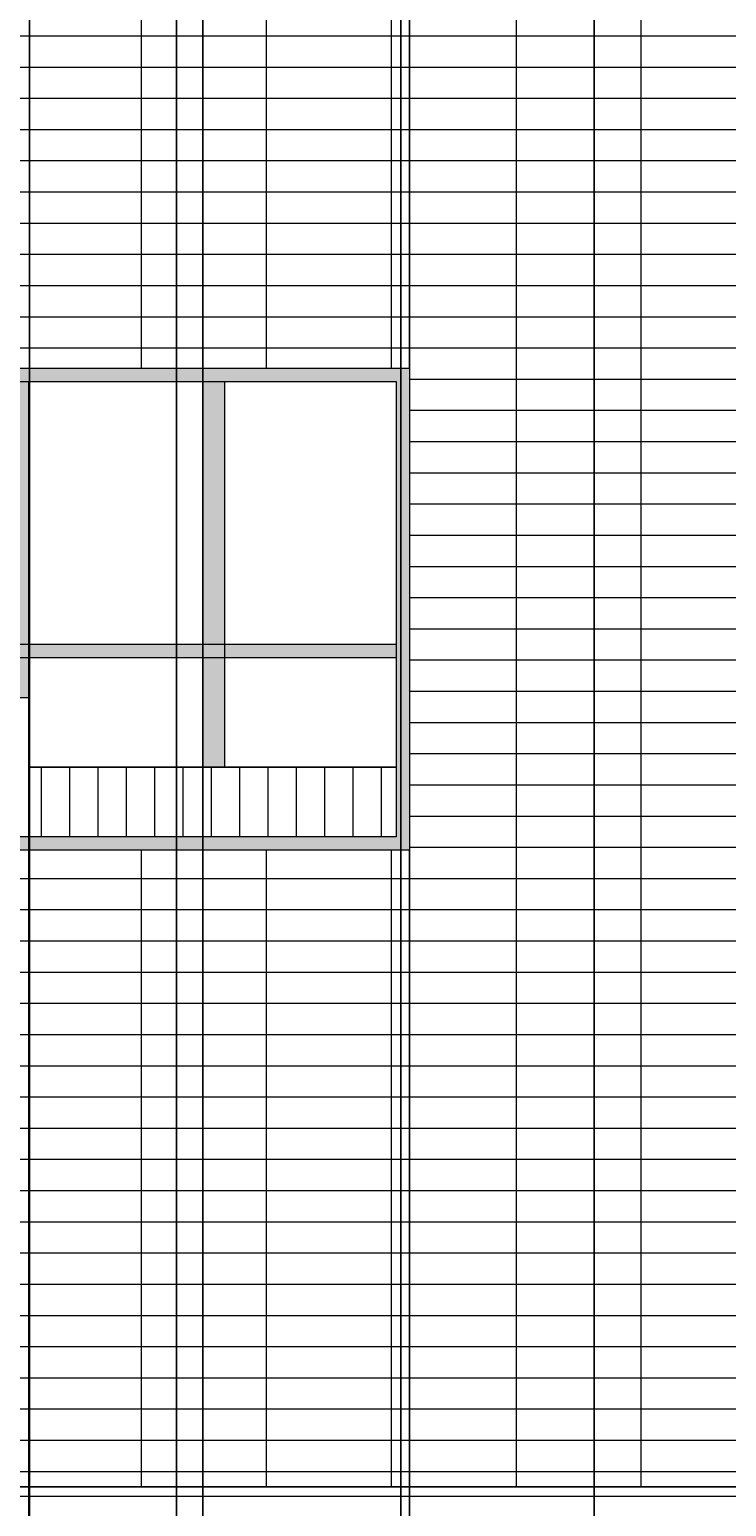
# Model space of a CAD drawing. Units: inches. Extents: x 241 to 943, y 109 to 1396.
# Tile 8 of 34: x 508 to 613, y 398 to 620. Entities that reach past the tile are written whole.
import ezdxf

# ---------------------------------------------------------------- set-up
doc = ezdxf.new("R2010")
doc.units = ezdxf.units.IN
doc.header["$MEASUREMENT"] = 0
for name, color, linetype, lineweight in [('A-ANNO-DIMS', 2, 'Continuous', 18), ('A-ELEV', 7, 'Continuous', 25), ('A-ELEV-SHAD', 9, 'Continuous', 13), ('A-GLAZ', 4, 'Continuous', 18), ('A-GLAZ-PATT', 18, 'Continuous', 13), ('A-WALL-PATT', 8, 'Continuous', 13)]:
    doc.layers.add(name, color=color, linetype=linetype, lineweight=lineweight)
doc.styles.get("Standard").update_dxf_attribs({"font": 'arial.ttf'})
doc.dimstyles.get("Standard").update_dxf_attribs({"dimtxt": 1.4375, "dimasz": 0.18, "dimexe": 0.18, "dimexo": 0.0625, "dimgap": 0.09, "dimtad": 0, "dimtih": 1, "dimtoh": 1, "dimdec": 4, "dimzin": 0, "dimdsep": 46, "dimlunit": 4, "dimtxsty": 'Standard', "dimcen": 0.09, "dimadec": 0, "dimazin": 0, "dimtfac": 1, "dimtdec": 4, "dimtofl": 0, "dimtmove": 0, "dimatfit": 3, "dimfxl": 1, "dimtolj": 1, "dimtzin": 0, "dimarcsym": 0})

# ---------------------------------------------------------------- blocks, each defined once
blk = doc.blocks.new('*D7')
at = {"layer": 'A-ANNO-DIMS', "color": 0, "lineweight": -2, "transparency": 16777216}
for p, q in [((508.24, 1336.12), (244.31, 1336.12)), ((244.49, 1335.94), (244.49, 753.25)), ((244.49, 168.92), (244.49, 751.6)), ((303.17, 168.74), (244.31, 168.74))]:
    blk.add_line(p, q, dxfattribs=at)
at = {"layer": 'A-ANNO-DIMS', "color": 0, "transparency": 16777216}
for points in [[(244.46, 1335.94), (244.52, 1335.94), (244.49, 1336.12)], [(244.46, 168.92), (244.52, 168.92), (244.49, 168.74)]]:
    blk.add_solid(points, dxfattribs=at)
at = {"layer": 'Defpoints', "color": 0, "transparency": 16777216}
for p in [(244.49, 1336.12), (508.31, 1336.12), (303.24, 168.74)]:
    blk.add_point(p, dxfattribs=at)
at = {"layer": 'A-ANNO-DIMS', "color": 0, "transparency": 16777216, "insert": (244.49, 752.43), "char_height": 1.438, "attachment_point": 5}
blk.add_mtext('\\A1;1167.4', dxfattribs=at)
blk = doc.blocks.new('*D11')
at = {"layer": 'A-ANNO-DIMS', "color": 0, "lineweight": -2, "transparency": 16777216}
for p, q in [((500.33, 384.24), (500.33, 1395.05)), ((500.51, 1394.87), (513.31, 1394.87)), ((530.05, 1394.87), (517.25, 1394.87)), ((530.23, 384.24), (530.23, 1395.05))]:
    blk.add_line(p, q, dxfattribs=at)
at = {"layer": 'A-ANNO-DIMS', "color": 0, "transparency": 16777216}
for points in [[(500.51, 1394.9), (500.51, 1394.84), (500.33, 1394.87)], [(530.05, 1394.9), (530.05, 1394.84), (530.23, 1394.87)]]:
    blk.add_solid(points, dxfattribs=at)
at = {"layer": 'Defpoints', "color": 0, "transparency": 16777216}
for p in [(530.23, 1394.87), (500.33, 384.18), (530.23, 384.18)]:
    blk.add_point(p, dxfattribs=at)
at = {"layer": 'A-ANNO-DIMS', "color": 0, "transparency": 16777216, "insert": (515.28, 1394.87), "char_height": 1.438, "attachment_point": 5}
blk.add_mtext('\\A1;29.9', dxfattribs=at)
blk = doc.blocks.new('*D12')
at = {"layer": 'A-ANNO-DIMS', "color": 0, "lineweight": -2, "transparency": 16777216}
for p, q in [((530.23, 384.24), (530.23, 1395.05)), ((530.41, 1394.87), (587.56, 1394.87)), ((650.73, 1394.87), (593.58, 1394.87)), ((650.91, 384.24), (650.91, 1395.05))]:
    blk.add_line(p, q, dxfattribs=at)
at = {"layer": 'A-ANNO-DIMS', "color": 0, "transparency": 16777216}
for points in [[(530.41, 1394.9), (530.41, 1394.84), (530.23, 1394.87)], [(650.73, 1394.9), (650.73, 1394.84), (650.91, 1394.87)]]:
    blk.add_solid(points, dxfattribs=at)
at = {"layer": 'Defpoints', "color": 0, "transparency": 16777216}
for p in [(650.91, 1394.87), (530.23, 384.18), (650.91, 384.18)]:
    blk.add_point(p, dxfattribs=at)
at = {"layer": 'A-ANNO-DIMS', "color": 0, "transparency": 16777216, "insert": (590.57, 1394.87), "char_height": 1.438, "attachment_point": 5}
blk.add_mtext('\\A1;120.68', dxfattribs=at)
blk = doc.blocks.new('*D41')
at = {"layer": 'A-ANNO-DIMS', "color": 0, "lineweight": -2, "transparency": 16777216}
for p, q in [((820.77, 400.83), (244.31, 400.83)), ((244.49, 400.65), (244.49, 317.65)), ((244.49, 233.01), (244.49, 316.01)), ((820.77, 232.83), (244.31, 232.83))]:
    blk.add_line(p, q, dxfattribs=at)
at = {"layer": 'A-ANNO-DIMS', "color": 0, "transparency": 16777216}
for points in [[(244.46, 400.65), (244.52, 400.65), (244.49, 400.83)], [(244.46, 233.01), (244.52, 233.01), (244.49, 232.83)]]:
    blk.add_solid(points, dxfattribs=at)
at = {"layer": 'Defpoints', "color": 0, "transparency": 16777216}
for p in [(244.49, 400.83), (820.84, 400.83), (820.84, 232.83)]:
    blk.add_point(p, dxfattribs=at)
at = {"layer": 'A-ANNO-DIMS', "color": 0, "transparency": 16777216, "insert": (244.49, 316.83), "char_height": 1.438, "attachment_point": 5}
blk.add_mtext('\\A1;168', dxfattribs=at)
blk = doc.blocks.new('*D62')
at = {"layer": 'A-ANNO-DIMS', "color": 0, "lineweight": -2, "transparency": 16777216}
for p, q in [((424.11, 568.89), (424.11, 1395.05)), ((424.29, 1394.87), (492.35, 1394.87)), ((565.02, 1394.87), (496.96, 1394.87)), ((565.2, 568.89), (565.2, 1395.05))]:
    blk.add_line(p, q, dxfattribs=at)
at = {"layer": 'A-ANNO-DIMS', "color": 0, "transparency": 16777216}
for points in [[(424.29, 1394.9), (424.29, 1394.84), (424.11, 1394.87)], [(565.02, 1394.9), (565.02, 1394.84), (565.2, 1394.87)]]:
    blk.add_solid(points, dxfattribs=at)
at = {"layer": 'Defpoints', "color": 0, "transparency": 16777216}
for p in [(565.2, 1394.87), (424.11, 568.83), (565.2, 568.83)]:
    blk.add_point(p, dxfattribs=at)
at = {"layer": 'A-ANNO-DIMS', "color": 0, "transparency": 16777216, "insert": (494.66, 1394.87), "char_height": 1.438, "attachment_point": 5}
blk.add_mtext('\\A1;141.1', dxfattribs=at)
blk = doc.blocks.new('*D82')
at = {"layer": 'A-ANNO-DIMS', "color": 0, "lineweight": -2, "transparency": 16777216}
for p, q in [((565.2, 568.89), (565.2, 1395.05)), ((565.38, 1394.87), (605.89, 1394.87)), ((651.42, 1394.87), (610.91, 1394.87)), ((651.6, 568.89), (651.6, 1395.05))]:
    blk.add_line(p, q, dxfattribs=at)
at = {"layer": 'A-ANNO-DIMS', "color": 0, "transparency": 16777216}
for points in [[(565.38, 1394.9), (565.38, 1394.84), (565.2, 1394.87)], [(651.42, 1394.9), (651.42, 1394.84), (651.6, 1394.87)]]:
    blk.add_solid(points, dxfattribs=at)
at = {"layer": 'Defpoints', "color": 0, "transparency": 16777216}
for p in [(651.6, 1394.87), (565.2, 568.83), (651.6, 568.83)]:
    blk.add_point(p, dxfattribs=at)
at = {"layer": 'A-ANNO-DIMS', "color": 0, "transparency": 16777216, "insert": (608.4, 1394.87), "char_height": 1.438, "attachment_point": 5}
blk.add_mtext('\\A1;86.40', dxfattribs=at)
blk = doc.blocks.new('*D99')
at = {"layer": 'A-ANNO-DIMS', "color": 0, "lineweight": -2, "transparency": 16777216}
for p, q in [((417.09, 181.71), (417.09, 1395.05)), ((417.27, 1394.87), (539.16, 1394.87)), ((667.21, 1394.87), (545.33, 1394.87)), ((667.39, 214.58), (667.39, 1395.05))]:
    blk.add_line(p, q, dxfattribs=at)
at = {"layer": 'A-ANNO-DIMS', "color": 0, "transparency": 16777216}
for points in [[(417.27, 1394.9), (417.27, 1394.84), (417.09, 1394.87)], [(667.21, 1394.9), (667.21, 1394.84), (667.39, 1394.87)]]:
    blk.add_solid(points, dxfattribs=at)
at = {"layer": 'Defpoints', "color": 0, "transparency": 16777216}
for p in [(667.39, 1394.87), (667.39, 214.52), (417.09, 181.65)]:
    blk.add_point(p, dxfattribs=at)
at = {"layer": 'A-ANNO-DIMS', "color": 0, "transparency": 16777216, "insert": (542.24, 1394.87), "char_height": 1.438, "attachment_point": 5}
blk.add_mtext('\\A1;250.30', dxfattribs=at)
blk = doc.blocks.new('*D128')
at = {"layer": 'A-ANNO-DIMS', "color": 0, "lineweight": -2, "transparency": 16777216}
for p, q in [((534.18, 651.27), (534.18, 109.81)), ((508.19, 630.34), (508.19, 109.81)), ((508.37, 109.99), (518.1, 109.99)), ((534, 109.99), (524.27, 109.99))]:
    blk.add_line(p, q, dxfattribs=at)
at = {"layer": 'A-ANNO-DIMS', "color": 0, "transparency": 16777216}
for points in [[(508.37, 110.02), (508.37, 109.96), (508.19, 109.99)], [(534, 110.02), (534, 109.96), (534.18, 109.99)]]:
    blk.add_solid(points, dxfattribs=at)
at = {"layer": 'Defpoints', "color": 0, "transparency": 16777216}
for p in [(534.18, 651.34), (508.19, 630.4), (534.18, 109.99)]:
    blk.add_point(p, dxfattribs=at)
at = {"layer": 'A-ANNO-DIMS', "color": 0, "transparency": 16777216, "insert": (521.18, 109.99), "char_height": 1.438, "attachment_point": 5}
blk.add_mtext('\\A1;25.987', dxfattribs=at)
blk = doc.blocks.new('*D129')
at = {"layer": 'A-ANNO-DIMS', "color": 0, "lineweight": -2, "transparency": 16777216}
for p, q in [((534.18, 651.27), (534.18, 109.81)), ((563.93, 651.27), (563.93, 109.81)), ((534.36, 109.99), (546.52, 109.99)), ((563.75, 109.99), (551.59, 109.99))]:
    blk.add_line(p, q, dxfattribs=at)
at = {"layer": 'A-ANNO-DIMS', "color": 0, "transparency": 16777216}
for points in [[(534.36, 110.02), (534.36, 109.96), (534.18, 109.99)], [(563.75, 110.02), (563.75, 109.96), (563.93, 109.99)]]:
    blk.add_solid(points, dxfattribs=at)
at = {"layer": 'Defpoints', "color": 0, "transparency": 16777216}
for p in [(534.18, 651.34), (563.93, 651.34), (563.93, 109.99)]:
    blk.add_point(p, dxfattribs=at)
at = {"layer": 'A-ANNO-DIMS', "color": 0, "transparency": 16777216, "insert": (549.05, 109.99), "char_height": 1.438, "attachment_point": 5}
blk.add_mtext('\\A1;29.75', dxfattribs=at)
blk = doc.blocks.new('*D130')
at = {"layer": 'A-ANNO-DIMS', "color": 0, "lineweight": -2, "transparency": 16777216}
for p, q in [((563.93, 651.27), (563.93, 109.81)), ((592.95, 628.34), (592.95, 109.81)), ((564.11, 109.99), (575.35, 109.99)), ((592.77, 109.99), (581.53, 109.99))]:
    blk.add_line(p, q, dxfattribs=at)
at = {"layer": 'A-ANNO-DIMS', "color": 0, "transparency": 16777216}
for points in [[(564.11, 110.02), (564.11, 109.96), (563.93, 109.99)], [(592.77, 110.02), (592.77, 109.96), (592.95, 109.99)]]:
    blk.add_solid(points, dxfattribs=at)
at = {"layer": 'Defpoints', "color": 0, "transparency": 16777216}
for p in [(563.93, 651.34), (592.95, 628.4), (592.95, 109.99)]:
    blk.add_point(p, dxfattribs=at)
at = {"layer": 'A-ANNO-DIMS', "color": 0, "transparency": 16777216, "insert": (578.44, 109.99), "char_height": 1.438, "attachment_point": 5}
blk.add_mtext('\\A1;29.025', dxfattribs=at)
blk = doc.blocks.new('*D138')
at = {"layer": 'A-ANNO-DIMS', "color": 0, "lineweight": -2, "transparency": 16777216}
for p, q in [((508.08, 508.84), (508.08, 109.81)), ((534.18, 508.84), (534.18, 109.81)), ((508.26, 109.99), (518.6, 109.99)), ((534, 109.99), (523.65, 109.99))]:
    blk.add_line(p, q, dxfattribs=at)
at = {"layer": 'A-ANNO-DIMS', "color": 0, "transparency": 16777216}
for points in [[(508.26, 110.02), (508.26, 109.96), (508.08, 109.99)], [(534, 110.02), (534, 109.96), (534.18, 109.99)]]:
    blk.add_solid(points, dxfattribs=at)
at = {"layer": 'Defpoints', "color": 0, "transparency": 16777216}
for p in [(508.08, 508.91), (534.18, 508.91), (534.18, 109.99)]:
    blk.add_point(p, dxfattribs=at)
at = {"layer": 'A-ANNO-DIMS', "color": 0, "transparency": 16777216, "insert": (521.13, 109.99), "char_height": 1.438, "attachment_point": 5}
blk.add_mtext('\\A1;26.10', dxfattribs=at)
blk = doc.blocks.new('*D139')
at = {"layer": 'A-ANNO-DIMS', "color": 0, "lineweight": -2, "transparency": 16777216}
for p, q in [((534.18, 508.84), (534.18, 109.81)), ((565.2, 496.38), (565.2, 109.81)), ((534.36, 109.99), (546.61, 109.99)), ((565.02, 109.99), (552.77, 109.99))]:
    blk.add_line(p, q, dxfattribs=at)
at = {"layer": 'A-ANNO-DIMS', "color": 0, "transparency": 16777216}
for points in [[(534.36, 110.02), (534.36, 109.96), (534.18, 109.99)], [(565.02, 110.02), (565.02, 109.96), (565.2, 109.99)]]:
    blk.add_solid(points, dxfattribs=at)
at = {"layer": 'Defpoints', "color": 0, "transparency": 16777216}
for p in [(534.18, 508.91), (565.2, 496.44), (565.2, 109.99)]:
    blk.add_point(p, dxfattribs=at)
at = {"layer": 'A-ANNO-DIMS', "color": 0, "transparency": 16777216, "insert": (549.69, 109.99), "char_height": 1.438, "attachment_point": 5}
blk.add_mtext('\\A1;31.025', dxfattribs=at)

msp = doc.modelspace()

# ---------------------------------------------------------------- hatches: boundary and pattern name
at = {"layer": 'A-ELEV-SHAD'}
h = msp.add_hatch(color=256, dxfattribs=at)
h.dxf.hatch_style = 1
h.paths.add_polyline_path([(537.4269, 566.8295), (534.1778, 566.8295), (534.1778, 527.3816), (537.4269, 527.3816)])
h.paths.add_polyline_path([(508.0803, 566.8295), (450.9259, 566.8295), (450.9259, 527.3816), (452.9259, 527.3816), (452.9259, 564.8295), (506.0803, 564.8295), (506.0803, 527.3816), (508.0803, 527.3816)])
h.paths.add_polyline_path([(481.5031, 564.8295), (479.5031, 564.8295), (479.5031, 527.3816), (481.5031, 527.3816)], flags=17)
h.paths.add_polyline_path([(481.5031, 525.3816), (479.5031, 525.3816), (479.5031, 521.3754), (481.5031, 521.3754)], flags=17)
h.paths.add_polyline_path([(508.0803, 525.3816), (506.0803, 525.3816), (506.0803, 521.3754), (452.9259, 521.3754), (452.9259, 525.3816), (450.9259, 525.3816), (450.9259, 519.3754), (508.0803, 519.3754)])
h.paths.add_polyline_path([(537.4269, 525.3816), (534.1778, 525.3816), (534.1778, 508.9074), (537.4269, 508.9074)])
h.paths.add_polyline_path([(749.6328, 702.7912), (617.7594, 702.7912), (617.7594, 700.7912), (747.6328, 700.7912), (747.6328, 628.4013), (617.7594, 628.4013), (617.7594, 626.4013), (749.6328, 626.4013)])
h.paths.add_polyline_path([(652.0129, 700.7912), (650.0129, 700.7912), (650.0129, 628.4013), (652.0129, 628.4013)], flags=17)
h.paths.add_polyline_path([(678.8698, 700.7912), (676.8698, 700.7912), (676.8698, 628.4013), (678.8698, 628.4013)], flags=17)
h.paths.add_polyline_path([(712.0171, 700.7912), (710.0171, 700.7912), (710.0171, 628.4013), (712.0171, 628.4013)], flags=17)
h.paths.add_polyline_path([(710.0171, 675.7856), (678.8698, 675.7856), (678.8698, 673.7856), (710.0171, 673.7856)], flags=17)
h.paths.add_polyline_path([(537.4269, 698.7912), (534.1778, 698.7912), (534.1778, 659.3434), (537.4269, 659.3434)], flags=0)
h.paths.add_polyline_path([(592.9542, 700.7912), (424.1086, 700.7912), (424.1086, 628.4013), (592.9542, 628.4013)])
h.paths.add_polyline_path([(590.8792, 698.7912), (590.8792, 630.4013), (426.1086, 630.4013), (426.1086, 698.7912)], flags=16)
h.paths.add_polyline_path([(563.2023, 698.7912), (563.2023, 659.3434), (563.9297, 659.3434), (563.9297, 651.3371), (508.1906, 651.3371), (508.0803, 651.3371), (450.9259, 651.3371), (428.0291, 651.3371), (428.0291, 698.7912), (451.9767, 698.7912), (508.0803, 698.7912), (537.4269, 698.7912)], flags=0)
h.paths.add_polyline_path([(506.0803, 696.7912), (506.0803, 653.3371), (452.9259, 653.3371), (452.9259, 657.3434), (445.5808, 657.3434, -1), (445.5808, 659.3434), (452.9259, 659.3434), (452.9259, 696.7912)], flags=0)
h.paths.add_polyline_path([(563.9297, 698.7912), (563.2023, 698.7912), (563.2023, 659.3434), (563.9297, 659.3434)], flags=0)
h = msp.add_hatch(color=256, dxfattribs=at)
h.dxf.hatch_style = 1
h.paths.add_polyline_path([(748.3325, 566.8295), (746.3325, 566.8295), (746.3325, 498.4395), (748.3325, 498.4395)])
h.paths.add_polyline_path([(746.3325, 524.3723), (691.794, 524.3723), (691.794, 522.3723), (746.3325, 522.3723)])
h.paths.add_polyline_path([(691.794, 566.8295), (689.794, 566.8295), (689.794, 498.4395), (691.794, 498.4395)])
h.paths.add_polyline_path([(790.691, 542.7994), (748.3325, 542.7994), (748.3325, 540.7994), (790.691, 540.7994)])
h.paths.add_polyline_path([(500.3323, 384.1784), (479.596, 384.1784), (479.596, 289.6933), (500.3323, 289.6933)])
h.paths.add_polyline_path([(481.596, 291.6933), (481.596, 382.1784), (498.3323, 382.1784), (498.3323, 291.6933)], flags=16)
h.paths.add_polyline_path([(462.1074, 384.1784), (390.895, 384.1784), (390.895, 289.6933), (462.1074, 289.6933)])
h.paths.add_polyline_path([(392.895, 291.6933), (392.895, 382.1784), (460.1074, 382.1784), (460.1074, 291.6933)], flags=16)
h.paths.add_polyline_path([(794.0275, 289.9984), (667.3935, 289.9984), (667.3935, 214.5189), (794.0275, 214.5189)])
h.paths.add_polyline_path([(792.0275, 287.9984), (792.0275, 216.5189), (669.3935, 216.5189), (669.3935, 287.9984)], flags=16)
h.paths.add_polyline_path([(508.0803, 525.3816), (506.0803, 525.3816), (506.0803, 521.3754), (452.9259, 521.3754), (452.9259, 525.3816), (450.9259, 525.3816), (450.9259, 519.3754), (508.0803, 519.3754)], flags=0)
h.paths.add_polyline_path([(508.0803, 566.8295), (450.9259, 566.8295), (450.9259, 527.3816), (452.9259, 527.3816), (452.9259, 564.8295), (506.0803, 564.8295), (506.0803, 527.3816), (508.0803, 527.3816)], flags=0)
h.paths.add_polyline_path([(537.4269, 566.8295), (534.1778, 566.8295), (534.1778, 527.3816), (537.4269, 527.3816)], flags=0)
h.paths.add_polyline_path([(537.4269, 525.3816), (534.1778, 525.3816), (534.1778, 508.9074), (537.4269, 508.9074)], flags=0)
h.paths.add_polyline_path([(565.2023, 568.8295), (424.1086, 568.8295), (424.1086, 496.4395), (565.2023, 496.4395)])
h.paths.add_polyline_path([(563.2023, 508.9074), (563.2023, 498.4395), (426.1086, 498.4395), (426.1086, 566.8295), (563.2023, 566.8295)], flags=16)
h.paths.add_polyline_path([(508.0803, 508.9074), (508.0803, 519.3754), (450.9259, 519.3754), (450.9259, 525.3816), (445.5808, 525.3816, -1), (445.5808, 527.3816), (450.9259, 527.3816), (450.9259, 566.8295), (508.0803, 566.8295), (537.4269, 566.8295), (537.4269, 508.9074)], flags=0)
h.paths.add_polyline_path([(506.0803, 521.3754), (452.9259, 521.3754), (452.9259, 564.8295), (506.0803, 564.8295)], flags=0)
at = {"layer": 'A-GLAZ-PATT'}
h = msp.add_hatch(dxfattribs=at)
h.set_pattern_fill('ANSI31', color=256, scale=34, angle=45)
h.paths.add_polyline_path([(486.3418, 786.9154), (413.1187, 786.9154), (413.1187, 761.2284), (486.3418, 761.2284)])
h.paths.add_polyline_path([(486.3418, 954.9154), (413.1187, 954.9154), (413.1187, 929.2284), (486.3418, 929.2284)])
h.paths.add_polyline_path([(462.1074, 289.6933), (390.895, 289.6933), (390.895, 277.4626), (390.895, 274.3507), (462.1074, 274.3507), (462.1074, 277.4626)])
h.paths.add_polyline_path([(500.3323, 289.6933), (479.596, 289.6933), (479.596, 274.3507), (500.3323, 274.3507)])
h.paths.add_polyline_path([(450.9259, 566.8295), (426.1086, 566.8295), (426.1086, 498.4395), (446.4348, 498.4395), (446.4348, 519.3754), (450.9259, 519.3754), (450.9259, 525.3816), (445.5808, 525.3816, -1), (445.5808, 527.3816), (450.9259, 527.3816)])
h.paths.add_polyline_path([(563.2023, 508.9074), (534.1778, 508.9074), (508.1906, 508.9074), (508.1906, 498.4395), (563.2023, 498.4395)])
h.paths.add_polyline_path([(747.6328, 700.7912), (712.0171, 700.7912), (712.0171, 628.4013), (747.6328, 628.4013)])
h.paths.add_polyline_path([(446.4348, 643.7483), (426.1086, 643.7483), (426.1086, 630.4013), (446.4348, 630.4013)])
h.paths.add_polyline_path([(564.8076, 841.5382), (553.5166, 841.5382), (508.3064, 841.5382), (508.3064, 782.5808), (564.8076, 782.5808)])
h.paths.add_polyline_path([(564.8076, 780.5808), (508.3064, 780.5808), (508.3064, 773.4916), (564.8076, 773.4916)])
h.paths.add_polyline_path([(792.691, 762.5799), (759.6248, 762.5799), (759.6248, 736.9235), (759.6248, 734.8538), (792.691, 734.8538)])
h.paths.add_polyline_path([(564.8076, 1009.5382), (553.5166, 1009.5382), (508.3064, 1009.5382), (508.3064, 950.5808), (562.3033, 950.5808, -1), (562.3033, 948.5808), (508.3064, 948.5808), (508.3064, 941.4916), (564.8076, 941.4916)])
h.paths.add_polyline_path([(486.3418, 1122.9154), (413.1187, 1122.9154), (413.1187, 1097.2284), (486.3418, 1097.2284)])
h = msp.add_hatch(color=256, dxfattribs=at)
h.dxf.hatch_style = 1
h.paths.add_polyline_path([(396.3125, 1118.5808), (390.5597, 1118.5808), (388.0428, 1118.5808, 1), (388.0428, 1116.5808), (390.5597, 1116.5808), (396.3125, 1116.5808)])
h.paths.add_polyline_path([(398.3125, 1118.5808), (396.3125, 1118.5808), (396.3125, 1116.5808), (398.3125, 1116.5808)])
h.paths.add_polyline_path([(413.1187, 1118.5808), (398.3125, 1118.5808), (398.3125, 1116.5808), (413.1187, 1116.5808)])
h.paths.add_polyline_path([(506.3064, 1118.5808), (486.3418, 1118.5808), (486.3418, 1116.5808), (506.3064, 1116.5808)])
h.paths.add_polyline_path([(506.8039, 1118.5808), (506.3064, 1118.5808), (506.3064, 1116.5808), (506.8039, 1116.5808, 1)])
h.paths.add_polyline_path([(396.3125, 950.5808), (390.5597, 950.5808), (388.0428, 950.5808, 1), (388.0428, 948.5808), (390.5597, 948.5808), (396.3125, 948.5808)])
h.paths.add_polyline_path([(398.3125, 950.5808), (396.3125, 950.5808), (396.3125, 948.5808), (398.3125, 948.5808)])
h.paths.add_polyline_path([(413.1187, 950.5808), (398.3125, 950.5808), (398.3125, 948.5808), (413.1187, 948.5808)])
h.paths.add_polyline_path([(506.3064, 950.5808), (486.3418, 950.5808), (486.3418, 948.5808), (506.3064, 948.5808)])
h.paths.add_polyline_path([(508.3064, 950.5808), (506.3064, 950.5808), (506.3064, 948.5808), (508.3064, 948.5808)])
h.paths.add_polyline_path([(562.3033, 950.5808), (508.3064, 950.5808), (508.3064, 948.5808), (562.3033, 948.5808, 1)])
h.paths.add_polyline_path([(396.3125, 782.5808), (390.5597, 782.5808), (388.0428, 782.5808, 1), (388.0428, 780.5808), (390.5597, 780.5808), (396.3125, 780.5808)])
h.paths.add_polyline_path([(398.3125, 782.5808), (396.3125, 782.5808), (396.3125, 780.5808), (398.3125, 780.5808)])
h.paths.add_polyline_path([(413.1187, 782.5808), (398.3125, 782.5808), (398.3125, 780.5808), (413.1187, 780.5808)])
h.paths.add_polyline_path([(506.3064, 782.5808), (486.3418, 782.5808), (486.3418, 780.5808), (506.3064, 780.5808)])
h.paths.add_polyline_path([(508.3064, 782.5808), (506.3064, 782.5808), (506.3064, 780.5808), (508.3064, 780.5808)])
h.paths.add_polyline_path([(564.8076, 782.5808), (508.3064, 782.5808), (508.3064, 780.5808), (564.8076, 780.5808)])
h.paths.add_polyline_path([(605.9087, 782.5808), (564.8076, 782.5808), (564.8076, 780.5808), (605.9087, 780.5808, 1)])
h.paths.add_polyline_path([(450.9259, 659.3434), (445.5808, 659.3434, 1), (445.5808, 657.3434), (450.9259, 657.3434)])
h.paths.add_polyline_path([(452.9259, 659.3434), (450.9259, 659.3434), (450.9259, 657.3434), (452.9259, 657.3434)])
h.paths.add_polyline_path([(506.0803, 659.3434), (452.9259, 659.3434), (452.9259, 657.3434), (506.0803, 657.3434)])
h.paths.add_polyline_path([(508.0803, 659.3434), (506.0803, 659.3434), (506.0803, 657.3434), (508.0803, 657.3434)])
h.paths.add_polyline_path([(563.2023, 659.3434), (537.4269, 659.3434), (537.4269, 657.3434), (563.2023, 657.3434)])
h.paths.add_polyline_path([(590.8792, 659.3434), (563.9297, 659.3434), (563.9297, 657.3434), (590.8792, 657.3434)])
h.paths.add_polyline_path([(563.9297, 659.3434), (563.2023, 659.3434), (563.2023, 657.3434), (563.9297, 657.3434)])
h.paths.add_polyline_path([(537.4269, 659.3434), (534.1778, 659.3434), (534.1778, 657.3434), (537.4269, 657.3434)])
h.paths.add_polyline_path([(534.1778, 659.3434), (508.0803, 659.3434), (508.0803, 657.3434), (534.1778, 657.3434)])
h.paths.add_polyline_path([(450.9259, 527.3816), (445.5808, 527.3816, 1), (445.5808, 525.3816), (450.9259, 525.3816)])
h.paths.add_polyline_path([(452.9259, 527.3816), (450.9259, 527.3816), (450.9259, 525.3816), (452.9259, 525.3816)])
h.paths.add_polyline_path([(479.5031, 527.3816), (452.9259, 527.3816), (452.9259, 525.3816), (479.5031, 525.3816)])
h.paths.add_polyline_path([(481.5031, 527.3816), (479.5031, 527.3816), (479.5031, 525.3816), (481.5031, 525.3816)])
h.paths.add_polyline_path([(506.0803, 527.3816), (481.5031, 527.3816), (481.5031, 525.3816), (506.0803, 525.3816)])
h.paths.add_polyline_path([(508.0803, 527.3816), (506.0803, 527.3816), (506.0803, 525.3816), (508.0803, 525.3816)])
h.paths.add_polyline_path([(563.2023, 527.3816), (508.0803, 527.3816), (508.0803, 525.3816), (563.2023, 525.3816)])
at = {"layer": 'A-WALL-PATT'}
h = msp.add_hatch(dxfattribs=at)
h.set_pattern_fill('GRATE', color=256, scale=150)
h.paths.add_polyline_path([(747.7579, 1238.8538), (747.7579, 1275.9142), (747.7579, 1336.1154), (508.3064, 1336.1154), (508.3064, 1275.9142), (508.3064, 1238.8538), (508.3064, 1177.5382), (508.3064, 1109.4916), (508.3064, 1070.8538), (553.5166, 1070.8538), (749.6328, 1070.8538)])
h.paths.add_polyline_path([(533.952, 1108.1686), (533.952, 1177.7336), (533.952, 1303.0286), (724.819, 1303.0286), (724.819, 1108.1686)], flags=16)
h.paths.add_polyline_path([(535.952, 1110.1686), (535.952, 1175.7336), (722.819, 1175.7336), (722.819, 1110.1686)], flags=0)
h.paths.add_polyline_path([(643.4534, 1134.0739), (622.521, 1134.0739), (622.521, 1136.0739), (643.4534, 1136.0739)], flags=0)
h.paths.add_polyline_path([(617.7594, 568.8295), (617.7594, 734.8538), (377.0391, 734.8538), (377.0391, 566.8538), (377.0391, 400.8295), (417.0913, 400.8295), (618.9643, 400.8295)])
h.paths.add_polyline_path([(424.1086, 496.4395), (424.1086, 568.8295), (565.2023, 568.8295), (565.2023, 496.4395)], flags=16)
h.paths.add_polyline_path([(426.1086, 498.4395), (426.1086, 566.8295), (563.2023, 566.8295), (563.2023, 508.9074), (563.2023, 498.4395)], flags=0)
h.paths.add_polyline_path([(508.0803, 508.9074), (508.0803, 519.3754), (450.9259, 519.3754), (450.9259, 525.3816), (445.5808, 525.3816, -1), (445.5808, 527.3816), (450.9259, 527.3816), (450.9259, 566.8295), (508.0803, 566.8295), (537.4269, 566.8295), (537.4269, 508.9074)], flags=0)
h.paths.add_polyline_path([(506.0803, 521.3754), (452.9259, 521.3754), (452.9259, 564.8295), (506.0803, 564.8295)], flags=0)
h.paths.add_polyline_path([(424.1086, 628.4013), (424.1086, 700.7912), (592.9542, 700.7912), (592.9542, 628.4013)], flags=16)
h.paths.add_polyline_path([(426.1086, 630.4013), (426.1086, 698.7912), (590.8792, 698.7912), (590.8792, 630.4013)], flags=0)
h.paths.add_polyline_path([(508.1906, 651.3371), (508.0803, 651.3371), (450.9259, 651.3371), (428.0291, 651.3371), (428.0291, 698.7912), (451.9767, 698.7912), (508.0803, 698.7912), (537.4269, 698.7912), (563.2023, 698.7912), (563.2023, 659.3434), (563.9297, 659.3434), (563.9297, 651.3371)], flags=0)
h.paths.add_polyline_path([(506.0803, 653.3371), (452.9259, 653.3371), (452.9259, 657.3434), (445.5808, 657.3434, -1), (445.5808, 659.3434), (452.9259, 659.3434), (452.9259, 696.7912), (506.0803, 696.7912)], flags=0)
h = msp.add_hatch(dxfattribs=at)
h.set_pattern_fill('GRATE', color=256, scale=150)
h.paths.add_polyline_path([(820.8374, 1070.8538), (749.6328, 1070.8538), (553.5166, 1070.8538), (508.3064, 1070.8538), (508.3064, 1009.5382), (553.5166, 1009.5382), (564.8076, 1009.5382), (603.8694, 1009.5382), (751.5078, 1009.5382), (751.5078, 902.8538), (603.8694, 902.8538), (603.8694, 1009.5382), (564.8076, 1009.5382), (564.8076, 941.4916), (568.1348, 941.4916), (568.1348, 902.8538), (581.3632, 902.8538), (581.3632, 841.5382), (564.8076, 841.5382), (564.8076, 782.5808), (605.9087, 782.5808, -1), (605.9087, 780.5808), (564.8076, 780.5808), (564.8076, 773.4916), (597.514, 773.4916), (607.8162, 773.4916), (607.8162, 734.8538), (617.7594, 734.8538), (617.7594, 841.5382), (792.691, 841.5382), (792.691, 734.8538), (617.7594, 734.8538), (617.7594, 702.7912), (749.6328, 702.7912), (749.6328, 626.4013), (617.7594, 626.4013), (617.7594, 568.8295), (820.8374, 568.8295), (820.8374, 736.8295), (820.8374, 902.8538)])
h = msp.add_hatch(dxfattribs=at)
h.set_pattern_fill('ANSI32', color=256, scale=71, angle=135)
h.paths.add_polyline_path([(820.8374, 568.8295), (792.691, 568.8295), (792.691, 496.4395), (651.5974, 496.4395), (651.5974, 568.8295), (617.7594, 568.8295), (618.9643, 400.8295), (417.0913, 400.8295), (377.0391, 400.8295), (377.0391, 398.8538), (377.0391, 396.8782), (377.0391, 228.8782), (377.0391, 177.6977), (416.5078, 181.5724), (417.0913, 181.649), (530.2303, 196.5065), (530.2303, 384.1784), (650.907, 384.1784), (651.7861, 212.4693), (667.3935, 214.5189), (667.3935, 289.9984), (794.0275, 289.9984), (794.0275, 232.8295), (820.8374, 232.8295), (820.8374, 400.8295)])
h.paths.add_polyline_path([(500.3323, 384.1784), (500.3323, 289.6933), (500.3323, 274.3507), (479.596, 274.3507), (479.596, 289.6933), (479.596, 384.1784)], flags=16)
h.paths.add_polyline_path([(498.3323, 382.1784), (498.3323, 291.6933), (481.596, 291.6933), (481.596, 382.1784)], flags=0)
h.paths.add_polyline_path([(462.1074, 384.1784), (462.1074, 289.6933), (462.1074, 277.4626), (462.1074, 274.3507), (390.895, 274.3507), (390.895, 277.4626), (390.895, 289.6933), (390.895, 384.1784)], flags=16)
h.paths.add_polyline_path([(460.1074, 382.1784), (460.1074, 291.6933), (392.895, 291.6933), (392.895, 382.1784)], flags=0)
h.paths.add_polyline_path([(595.3136, 372.9401), (641.6196, 372.9401), (641.6196, 246.4081), (651.6121, 246.4593), (650.907, 384.1784), (530.2303, 384.1784), (530.2303, 245.8378), (595.3136, 246.1711)], flags=17)

# ---------------------------------------------------------------- linework, layer by layer
at = {"layer": 'A-ELEV'}
msp.add_line((417.0913, 400.8295), (618.9643, 400.8295), dxfattribs=at)
at = {"layer": 'A-GLAZ'}
for p, q in [((445.5808, 527.3816), (563.2023, 527.3816)), ((445.5808, 525.3816), (563.2023, 525.3816)), ((446.4348, 519.3754), (508.1906, 519.3754)), ((508.1906, 519.3754), (508.1906, 498.4395)), ((508.1906, 508.9074), (563.2023, 508.9074))]:
    msp.add_line(p, q, dxfattribs=at)
for points in [[(424.1086, 568.8295), (565.2023, 568.8295), (565.2023, 496.4395), (424.1086, 496.4395)], [(426.1086, 566.8295), (563.2023, 566.8295), (563.2023, 498.4395), (426.1086, 498.4395)], [(508.0803, 566.8295), (537.4269, 566.8295), (537.4269, 508.9074), (508.0803, 508.9074)], [(534.1778, 566.8295), (563.2023, 566.8295), (563.2023, 508.9074), (534.1778, 508.9074)]]:
    msp.add_lwpolyline(points, close=True, dxfattribs=at)

# ---------------------------------------------------------------- dimensions: what is measured, and where the dimension line sits
at = {"layer": 'A-ANNO-DIMS'}
for base, p1, p2, override, picture, middle in [((667.3935, 1394.8654), (417.0913, 181.649), (667.3935, 214.5189), {"dimdec": 2, "dimlfac": 1, "dimrnd": 0, "dimzin": 0, "dimdsep": 46, "dimlunit": 2}, '*D99', (542.2424, 1394.8654)), ((565.2023, 1394.8654), (424.1086, 568.8295), (565.2023, 568.8295), {"dimdec": 1, "dimlfac": 1, "dimrnd": 0, "dimzin": 0, "dimdsep": 46, "dimlunit": 2}, '*D62', (494.6554, 1394.8654)), ((530.2303, 1394.8654), (500.3323, 384.1784), (530.2303, 384.1784), {"dimdec": 1, "dimlfac": 1, "dimrnd": 0, "dimzin": 0, "dimdsep": 46, "dimlunit": 2}, '*D11', (515.2813, 1394.8654)), ((650.907, 1394.8654), (530.2303, 384.1784), (650.907, 384.1784), {"dimdec": 2, "dimlfac": 1, "dimrnd": 0, "dimzin": 0, "dimdsep": 46, "dimlunit": 2}, '*D12', (590.5686, 1394.8654)), ((651.5974, 1394.8654), (565.2023, 568.8295), (651.5974, 568.8295), {"dimdec": 2, "dimlfac": 1, "dimrnd": 0, "dimzin": 0, "dimdsep": 46, "dimlunit": 2}, '*D82', (608.3998, 1394.8654)), ((534.1778, 109.9907), (508.1906, 630.4013), (534.1778, 651.3371), {"dimdec": 3, "dimlfac": 1, "dimrnd": 0, "dimzin": 0, "dimdsep": 46, "dimlunit": 2}, '*D128', (521.1842, 109.9907)), ((563.9297, 109.9907), (534.1778, 651.3371), (563.9297, 651.3371), {"dimdec": 2, "dimlfac": 1, "dimrnd": 0, "dimzin": 0, "dimdsep": 46, "dimlunit": 2}, '*D129', (549.0538, 109.9907)), ((592.954223, 109.990742), (563.92972, 651.337109), (592.954223, 628.401255), {"dimdec": 3, "dimlfac": 1, "dimrnd": 0, "dimzin": 0, "dimdsep": 46, "dimlunit": 2}, '*D130', (578.441971, 109.990742)), ((534.1778, 109.9907), (508.0803, 508.9074), (534.1778, 508.9074), {"dimdec": 2, "dimlfac": 1, "dimrnd": 0, "dimzin": 0, "dimdsep": 46, "dimlunit": 2}, '*D138', (521.1291, 109.9907)), ((565.20229, 109.99074), (534.17778, 508.90744), (565.20229, 496.43952), {"dimdec": 3, "dimlfac": 1, "dimrnd": 0, "dimzin": 0, "dimdsep": 46, "dimlunit": 2}, '*D139', (549.69004, 109.99074))]:
    dim = msp.add_linear_dim(base=base, p1=p1, p2=p2, dimstyle='Standard', override=override, dxfattribs=at)
    dim.commit()
    dim.dimension.update_dxf_attribs({"geometry": picture, "text_midpoint": middle})
for base, p1, p2, override, picture, middle in [((244.4858, 1336.1154), (303.2358, 168.7407), (508.3064, 1336.1154), {"dimdec": 1, "dimlfac": 1, "dimrnd": 0, "dimzin": 0, "dimdsep": 46, "dimlunit": 2}, '*D7', (244.4858, 752.4281)), ((244.4858, 400.8295), (820.8374, 232.8295), (820.8374, 400.8295), {"dimdec": 0, "dimlfac": 1, "dimrnd": 0, "dimzin": 0, "dimdsep": 46, "dimlunit": 2}, '*D41', (244.4858, 316.8295))]:
    dim = msp.add_linear_dim(base=base, p1=p1, p2=p2, angle=90, dimstyle='Standard', override=override, dxfattribs=at)
    dim.commit()
    dim.dimension.update_dxf_attribs({"geometry": picture, "text_midpoint": middle})

doc.saveas('drawing.dxf')
